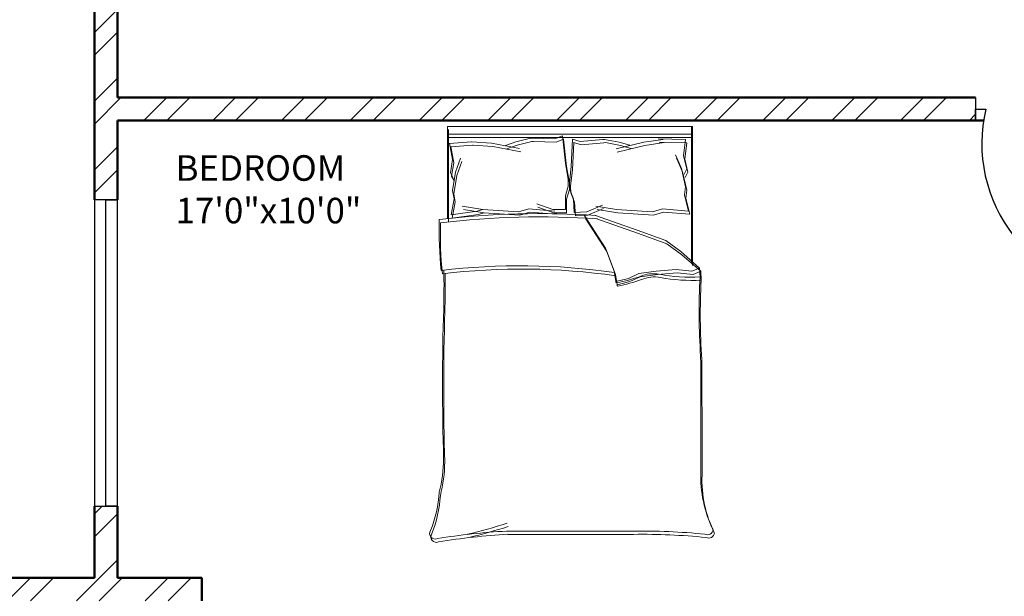
# Model space of a CAD drawing. Units: inches. Extents: x 963 to 2075, y 289 to 2657.
# Tile 60 of 98: x 1149 to 1342, y 2117 to 2230. Entities that reach past the tile are written whole.
import ezdxf

# ---------------------------------------------------------------- set-up
doc = ezdxf.new("R2010")
doc.units = ezdxf.units.IN
for name, color, linetype, lineweight in [('A-AREA-IDEN', 7, 'Continuous', 18), ('A-DOOR', 4, 'Continuous', 25), ('A-FURN', 8, 'Continuous', 18), ('A-GLAZ', 3, 'Continuous', 25), ('A-WALL', 7, 'Continuous', 50), ('A-WALL-PATT', 8, 'Continuous', 13)]:
    doc.layers.add(name, color=color, linetype=linetype, lineweight=lineweight)
doc.styles.get("Standard").update_dxf_attribs({"font": 'arial.ttf'})

# ---------------------------------------------------------------- blocks, each defined once
blk = doc.blocks.new('BED-DOUBLE')
for p, q in [((1236.76, 2450.75), (1254.87, 2450.75)), ((1236.76, 2450.75), (1254.87, 2450.75)), ((1253.34, 2450.75), (1253.34, 2402.96)), ((1253.34, 2450.75), (1253.34, 2402.96)), ((1254.87, 2450.75), (1254.87, 2402.73)), ((1236.12, 2450.52), (1254.23, 2450.52)), ((1236.12, 2450.52), (1254.23, 2450.52)), ((1237.61, 2444.71), (1236.89, 2449.81)), ((1236.89, 2449.81), (1240.07, 2449.23)), ((1237.61, 2444.71), (1236.89, 2449.81)), ((1236.89, 2449.81), (1240.07, 2449.23)), ((1238.25, 2444.94), (1237.53, 2450.04)), ((1237.53, 2450.04), (1240.71, 2449.46)), ((1238.25, 2444.94), (1237.53, 2450.04)), ((1237.53, 2450.04), (1240.71, 2449.46)), ((1240.07, 2449.23), (1241.66, 2449.52)), ((1240.07, 2449.23), (1241.66, 2449.52)), ((1240.71, 2449.46), (1242.3, 2449.75)), ((1240.71, 2449.46), (1242.3, 2449.75)), ((1241.66, 2449.52), (1245.28, 2448.94)), ((1241.66, 2449.52), (1245.28, 2448.94)), ((1242.3, 2449.75), (1245.92, 2449.17)), ((1242.3, 2449.75), (1245.92, 2449.17)), ((1245.13, 2449.96), (1244.12, 2449.38)), ((1245.13, 2449.96), (1244.12, 2449.38)), ((1245.77, 2450.18), (1244.76, 2449.61)), ((1245.77, 2450.18), (1244.76, 2449.61)), ((1247.74, 2449.52), (1245.13, 2449.96)), ((1247.74, 2449.52), (1245.13, 2449.96)), ((1245.28, 2448.94), (1248.02, 2447.93)), ((1245.28, 2448.94), (1248.02, 2447.93)), ((1248.37, 2449.75), (1245.77, 2450.18)), ((1248.37, 2449.75), (1245.77, 2450.18)), ((1245.92, 2449.17), (1248.66, 2448.16)), ((1245.92, 2449.17), (1248.66, 2448.16)), ((1250.92, 2450.1), (1247.74, 2449.52)), ((1250.92, 2450.1), (1247.74, 2449.52)), ((1251.56, 2450.33), (1248.37, 2449.75)), ((1251.56, 2450.33), (1248.37, 2449.75)), ((1250.89, 2450.1), (1251.22, 2445.82)), ((1250.89, 2450.1), (1251.22, 2445.82)), ((1251.53, 2450.32), (1251.86, 2446.04)), ((1251.53, 2450.32), (1251.86, 2446.04)), ((1252.7, 2450.52), (1252.7, 2402.73)), ((1252.7, 2450.52), (1252.7, 2402.73)), ((1238.6, 2447.61), (1237.94, 2443.58)), ((1238.6, 2447.61), (1237.94, 2443.58)), ((1239.24, 2447.84), (1238.58, 2443.81)), ((1239.24, 2447.84), (1238.58, 2443.81)), ((1238.58, 2443.81), (1238.25, 2444.94)), ((1238.58, 2443.81), (1238.25, 2444.94)), ((1251.21, 2445.71), (1250.92, 2441.89)), ((1251.21, 2445.71), (1250.92, 2441.89)), ((1251.22, 2445.82), (1251.21, 2445.71)), ((1251.22, 2445.82), (1251.21, 2445.71)), ((1251.84, 2445.94), (1251.56, 2442.11)), ((1251.84, 2445.94), (1251.56, 2442.11)), ((1251.86, 2446.04), (1251.84, 2445.94)), ((1251.86, 2446.04), (1251.84, 2445.94)), ((1237.94, 2443.58), (1237.51, 2436.57)), ((1237.94, 2443.58), (1237.51, 2436.57)), ((1237.94, 2443.58), (1237.61, 2444.71)), ((1237.94, 2443.58), (1237.61, 2444.71)), ((1238.58, 2443.81), (1238.15, 2436.8)), ((1238.58, 2443.81), (1238.15, 2436.8)), ((1250.92, 2441.89), (1249.9, 2436.39)), ((1250.92, 2441.89), (1249.9, 2436.39)), ((1251.56, 2442.11), (1250.54, 2436.62)), ((1251.56, 2442.11), (1250.54, 2436.62)), ((1175.63, 2439.16), (1175.63, 2414.55)), ((1175.63, 2439.16), (1175.63, 2414.55)), ((1250.48, 2439.14), (1251.21, 2437.12)), ((1250.48, 2439.14), (1251.21, 2437.12)), ((1251.12, 2439.37), (1251.84, 2437.34)), ((1251.12, 2439.37), (1251.84, 2437.34)), ((1174.99, 2438.93), (1174.99, 2414.32)), ((1174.99, 2438.93), (1174.99, 2414.32)), ((1251.21, 2437.12), (1251.93, 2434.22)), ((1251.21, 2437.12), (1251.93, 2434.23)), ((1251.84, 2437.34), (1252.57, 2434.45)), ((1251.84, 2437.34), (1252.57, 2434.45)), ((1237.51, 2436.57), (1238.06, 2434.61)), ((1237.51, 2436.57), (1238.06, 2434.61)), ((1238.15, 2436.8), (1238.7, 2434.84)), ((1238.15, 2436.8), (1238.7, 2434.84)), ((1238.06, 2434.61), (1237.66, 2429.48)), ((1238.06, 2434.61), (1237.66, 2429.48)), ((1238.7, 2434.84), (1238.3, 2429.71)), ((1238.7, 2434.84), (1238.3, 2429.71)), ((1238.61, 2430.12), (1239.7, 2433.26)), ((1238.61, 2430.12), (1239.7, 2433.26)), ((1251.93, 2433.9), (1251.78, 2429.46)), ((1251.93, 2433.9), (1251.78, 2429.46)), ((1251.93, 2434.23), (1251.93, 2433.9)), ((1251.93, 2434.22), (1251.93, 2433.9)), ((1252.57, 2434.13), (1252.42, 2429.69)), ((1252.57, 2434.13), (1252.42, 2429.69)), ((1252.57, 2434.45), (1252.57, 2434.13)), ((1252.57, 2434.45), (1252.57, 2434.13)), ((1237.97, 2429.89), (1239.06, 2433.04)), ((1237.97, 2429.89), (1239.06, 2433.04)), ((1237.97, 2427.43), (1237.97, 2429.89)), ((1237.97, 2427.43), (1237.97, 2429.89)), ((1238.61, 2427.66), (1238.61, 2430.12)), ((1238.61, 2427.66), (1238.61, 2430.12)), ((1251.78, 2429.46), (1252.36, 2428.01)), ((1251.78, 2429.46), (1252.36, 2428.01)), ((1252.42, 2429.69), (1253, 2428.24)), ((1252.42, 2429.69), (1253, 2428.24)), ((1240.65, 2427.43), (1237.97, 2427.43)), ((1240.65, 2427.43), (1237.97, 2427.43)), ((1241.29, 2427.66), (1238.61, 2427.66)), ((1241.29, 2427.66), (1238.61, 2427.66)), ((1242.53, 2426.86), (1240.65, 2427.43)), ((1242.53, 2426.86), (1240.65, 2427.43)), ((1243.17, 2427.08), (1241.29, 2427.66)), ((1243.17, 2427.08), (1241.29, 2427.66)), ((1247.01, 2427.43), (1243.83, 2426.86)), ((1247.01, 2427.43), (1243.83, 2426.86)), ((1247.65, 2427.66), (1244.47, 2427.08)), ((1247.65, 2427.66), (1244.47, 2427.08)), ((1252.36, 2428.01), (1247.01, 2427.43)), ((1252.36, 2428.01), (1247.01, 2427.43)), ((1253, 2428.24), (1247.65, 2427.66)), ((1253, 2428.24), (1247.65, 2427.66)), ((1240.02, 2425.86), (1237.34, 2425.7)), ((1240.02, 2425.86), (1237.34, 2425.7)), ((1237.34, 2425.7), (1237.49, 2423.24)), ((1237.34, 2425.7), (1237.49, 2423.24)), ((1240.66, 2426.09), (1237.98, 2425.93)), ((1240.66, 2426.09), (1237.98, 2425.93)), ((1237.98, 2425.93), (1238.13, 2423.47)), ((1237.98, 2425.93), (1238.13, 2423.47)), ((1241.86, 2426.56), (1240.02, 2425.86)), ((1241.86, 2426.56), (1240.02, 2425.86)), ((1242.49, 2426.79), (1240.66, 2426.09)), ((1242.49, 2426.79), (1240.66, 2426.09)), ((1243.15, 2426.64), (1241.86, 2426.56)), ((1243.15, 2426.64), (1241.86, 2426.56)), ((1243.79, 2426.87), (1242.49, 2426.79)), ((1243.79, 2426.87), (1242.49, 2426.79)), ((1243.83, 2426.86), (1242.53, 2426.86)), ((1243.83, 2426.86), (1242.53, 2426.86)), ((1246.37, 2426.26), (1243.15, 2426.64)), ((1246.37, 2426.26), (1243.15, 2426.64)), ((1244.47, 2427.08), (1243.17, 2427.08)), ((1244.47, 2427.08), (1243.17, 2427.08)), ((1247, 2426.49), (1243.79, 2426.87)), ((1247, 2426.49), (1243.79, 2426.87)), ((1251.74, 2426.02), (1246.37, 2426.26)), ((1251.74, 2426.02), (1246.37, 2426.26)), ((1252.38, 2426.25), (1247, 2426.49)), ((1252.38, 2426.25), (1247, 2426.49)), ((1251.25, 2424.54), (1251.74, 2426.02)), ((1251.25, 2424.54), (1251.74, 2426.02)), ((1251.89, 2424.77), (1252.38, 2426.25)), ((1251.89, 2424.77), (1252.38, 2426.25)), ((1236.85, 2423.74), (1230.36, 2419.55)), ((1236.85, 2423.74), (1230.36, 2419.55)), ((1237.49, 2423.96), (1231, 2419.77)), ((1237.49, 2423.96), (1231, 2419.77)), ((1251.68, 2420.11), (1251.25, 2424.54)), ((1251.68, 2420.11), (1251.25, 2424.54)), ((1252.31, 2420.34), (1251.89, 2424.77)), ((1252.31, 2420.34), (1251.89, 2424.77)), ((1233.92, 2413.35), (1236.85, 2421.69)), ((1233.92, 2413.35), (1236.85, 2421.69)), ((1234.56, 2413.58), (1237.49, 2421.92)), ((1234.56, 2413.58), (1237.49, 2421.92)), ((1237.49, 2423.24), (1238.78, 2420.17)), ((1237.49, 2423.24), (1238.78, 2420.17)), ((1238.13, 2423.47), (1239.42, 2420.4)), ((1238.13, 2423.47), (1239.42, 2420.4)), ((1239.24, 2421.66), (1238.58, 2417.63)), ((1239.24, 2421.66), (1238.58, 2417.63)), ((1231, 2419.77), (1226.51, 2418.07)), ((1231, 2419.77), (1226.51, 2418.07)), ((1238.6, 2421.43), (1237.94, 2417.4)), ((1238.6, 2421.43), (1237.94, 2417.4)), ((1251.15, 2416.86), (1251.7, 2419.79)), ((1251.15, 2416.86), (1251.7, 2419.79)), ((1251.7, 2419.79), (1251.68, 2420.11)), ((1251.7, 2419.79), (1251.68, 2420.11)), ((1251.79, 2417.09), (1252.33, 2420.02)), ((1251.79, 2417.09), (1252.33, 2420.02)), ((1252.33, 2420.02), (1252.31, 2420.34)), ((1252.33, 2420.02), (1252.31, 2420.34)), ((1225.87, 2417.84), (1223.86, 2417.53)), ((1225.87, 2417.84), (1223.86, 2417.53)), ((1226.51, 2418.07), (1224.49, 2417.76)), ((1226.51, 2418.07), (1224.49, 2417.76)), ((1230.36, 2419.55), (1225.87, 2417.84)), ((1230.36, 2419.55), (1225.87, 2417.84)), ((1223.86, 2417.53), (1224.47, 2415.05)), ((1223.86, 2417.53), (1224.47, 2415.05)), ((1224.49, 2417.76), (1225.11, 2415.28)), ((1224.49, 2417.76), (1225.11, 2415.28)), ((1237.94, 2417.4), (1237.51, 2410.39)), ((1237.94, 2417.4), (1237.51, 2410.39)), ((1238.58, 2417.63), (1238.15, 2410.62)), ((1238.58, 2417.63), (1238.15, 2410.62)), ((1251.16, 2412.08), (1249.81, 2417.5)), ((1251.16, 2412.08), (1249.81, 2417.5)), ((1251.8, 2412.31), (1250.45, 2417.73)), ((1251.8, 2412.31), (1250.45, 2417.73)), ((1250.56, 2414.79), (1251.15, 2416.86)), ((1250.56, 2414.79), (1251.15, 2416.86)), ((1251.2, 2415.02), (1251.79, 2417.09)), ((1251.2, 2415.02), (1251.79, 2417.09)), ((1224.47, 2415.05), (1225.4, 2413.04)), ((1224.47, 2415.05), (1225.4, 2413.04)), ((1225.11, 2415.28), (1226.04, 2413.27)), ((1225.11, 2415.28), (1226.04, 2413.27)), ((1225.4, 2413.04), (1225.87, 2409.63)), ((1225.4, 2413.04), (1225.87, 2409.63)), ((1226.04, 2413.27), (1226.51, 2409.86)), ((1226.04, 2413.27), (1226.51, 2409.86)), ((1231.9, 2407.77), (1233.92, 2413.35)), ((1231.9, 2407.78), (1233.92, 2413.35)), ((1232.54, 2408), (1234.56, 2413.58)), ((1232.54, 2408), (1234.56, 2413.58)), ((1251.69, 2408.28), (1251.16, 2412.08)), ((1251.69, 2408.28), (1251.16, 2412.08)), ((1252.33, 2408.51), (1251.8, 2412.31)), ((1252.33, 2408.51), (1251.8, 2412.31)), ((1237.51, 2410.39), (1238.06, 2408.43)), ((1237.51, 2410.39), (1238.06, 2408.43)), ((1238.15, 2410.62), (1238.7, 2408.66)), ((1238.15, 2410.62), (1238.7, 2408.66)), ((1225.87, 2409.63), (1226.18, 2405.76)), ((1225.87, 2409.63), (1226.18, 2405.76)), ((1226.51, 2409.86), (1226.82, 2405.99)), ((1226.51, 2409.86), (1226.82, 2405.99)), ((1238.06, 2408.43), (1237.66, 2403.3)), ((1238.06, 2408.43), (1237.66, 2403.3)), ((1238.7, 2408.66), (1238.3, 2403.52)), ((1238.7, 2408.66), (1238.3, 2403.52)), ((1251.68, 2403.88), (1251.77, 2409.29)), ((1251.68, 2403.88), (1251.77, 2409.28)), ((1251.77, 2409.29), (1251.69, 2408.28)), ((1251.77, 2409.28), (1251.69, 2408.28)), ((1252.31, 2404.11), (1252.41, 2409.51)), ((1252.31, 2404.11), (1252.41, 2409.51)), ((1252.41, 2409.51), (1252.33, 2408.51)), ((1252.41, 2409.51), (1252.33, 2408.51)), ((1229.74, 2404.83), (1231.9, 2407.78)), ((1229.74, 2404.83), (1231.9, 2407.77)), ((1230.38, 2405.06), (1232.54, 2408)), ((1230.38, 2405.06), (1232.54, 2408)), ((1226.18, 2405.76), (1225.87, 2402.66)), ((1226.18, 2405.76), (1225.87, 2402.66)), ((1226.49, 2401.13), (1229.74, 2404.83)), ((1226.49, 2401.13), (1229.74, 2404.83)), ((1226.82, 2405.99), (1226.51, 2402.89)), ((1226.82, 2405.99), (1226.51, 2402.89)), ((1227.13, 2401.36), (1230.38, 2405.06)), ((1227.13, 2401.36), (1230.38, 2405.06)), ((1238.3, 2403.52), (1241.44, 2404.3)), ((1238.3, 2403.52), (1241.44, 2404.3)), ((1241.44, 2404.3), (1243.04, 2404.11)), ((1241.44, 2404.3), (1243.04, 2404.11)), ((1242.4, 2403.88), (1245.98, 2404.69)), ((1242.4, 2403.88), (1245.98, 2404.69)), ((1243.04, 2404.11), (1246.61, 2404.91)), ((1243.04, 2404.11), (1246.61, 2404.91)), ((1246.53, 2403.89), (1245.49, 2404.41)), ((1246.53, 2403.89), (1245.49, 2404.41)), ((1245.98, 2404.69), (1248.65, 2405.87)), ((1245.98, 2404.69), (1248.65, 2405.87)), ((1249.1, 2404.49), (1246.53, 2403.89)), ((1249.1, 2404.49), (1246.53, 2403.89)), ((1246.61, 2404.91), (1249.29, 2406.1)), ((1246.61, 2404.91), (1249.29, 2406.09)), ((1252.31, 2404.11), (1249.1, 2404.49)), ((1252.31, 2404.11), (1249.1, 2404.49)), ((1225.87, 2402.66), (1226.49, 2401.13)), ((1225.87, 2402.66), (1226.49, 2401.13)), ((1226.51, 2402.89), (1227.13, 2401.36)), ((1226.51, 2402.89), (1227.13, 2401.36)), ((1254.23, 2402.73), (1227.62, 2402.73)), ((1254.23, 2402.73), (1227.62, 2402.73)), ((1254.87, 2402.96), (1228.26, 2402.96)), ((1254.87, 2402.96), (1228.26, 2402.96)), ((1237.66, 2403.3), (1240.8, 2404.07)), ((1237.66, 2403.3), (1240.8, 2404.07)), ((1240.8, 2404.07), (1242.4, 2403.88)), ((1240.8, 2404.07), (1242.4, 2403.88)), ((1245.89, 2403.67), (1244.85, 2404.18)), ((1245.89, 2403.67), (1244.85, 2404.18)), ((1248.46, 2404.26), (1245.89, 2403.67)), ((1248.46, 2404.26), (1245.89, 2403.67)), ((1251.68, 2403.88), (1248.46, 2404.26)), ((1251.68, 2403.88), (1248.46, 2404.26)), ((1254.87, 2402.73), (1254.23, 2402.73)), ((1224.74, 2401.05), (1226.49, 2401.13, 3.87)), ((1224.74, 2401.05), (1226.49, 2401.13, 3.87)), ((1225.38, 2401.28), (1227.13, 2401.36, 3.87)), ((1225.38, 2401.28), (1227.13, 2401.36, 3.87))]:
    blk.add_line(p, q)
for centre, radius, start, end in [((1174.51, 2452.91), 1.09, 56.1736, 203.4781), ((1174.51, 2452.91), 1.09, 56.1736, 203.4781), ((1053.4, 2432.57), 121.76, 2.9958, 9.4091), ((1053.4, 2432.57), 121.76, 2.9958, 9.4091), ((1175.15, 2453.14), 1.09, 56.1736, 203.4781), ((1175.15, 2453.14), 1.09, 56.1736, 203.4781), ((1054.03, 2432.8), 121.76, 2.9958, 9.4091), ((1054.03, 2432.8), 121.76, 2.9958, 9.4091), ((1183.96, 2475.65), 23.56, 247.9751, 266.652), ((1183.96, 2475.65), 23.56, 247.9751, 266.652), ((1184.6, 2475.88), 23.56, 247.9751, 266.652), ((1184.6, 2475.88), 23.56, 247.9751, 266.652), ((1189.72, 2480.89), 29.63, 256.0648, 268.9113), ((1189.72, 2480.89), 29.63, 256.0648, 268.9113), ((1190.36, 2481.12), 29.63, 256.0648, 268.9113), ((1190.36, 2481.12), 29.63, 256.0648, 268.9113), ((1203.62, 1969.17), 482.31, 88.2277, 91.7185), ((1203.62, 1969.17), 482.31, 88.2277, 91.7185), ((1204.26, 1969.4), 482.31, 88.2277, 91.7185), ((1204.26, 1969.4), 482.31, 88.2277, 91.7185), ((1223.06, 2621.3), 170.11, 268.4762, 271.0082), ((1223.06, 2621.3), 170.11, 268.4762, 271.0082), ((1223.7, 2621.53), 170.11, 268.4762, 271.0082), ((1223.7, 2621.53), 170.11, 268.4762, 271.0082), ((1097.92, 2436.24), 129.02, 351.7845, 6.9006), ((1097.92, 2436.24), 129.02, 351.7845, 6.9006), ((1234.14, 2368.83), 83.31, 88.7218, 95.604), ((1234.14, 2368.83), 83.31, 88.7218, 95.604), ((1098.56, 2436.47), 129.02, 351.7845, 6.9006), ((1098.56, 2436.47), 129.02, 351.7845, 6.9006), ((1234.78, 2369.06), 83.31, 88.7218, 95.604), ((1234.78, 2369.06), 83.31, 88.7218, 95.604), ((1072.18, 2432.64), 164.97, 356.0865, 6.7821), ((1072.18, 2432.64), 164.97, 356.0865, 6.7821), ((1072.82, 2432.86), 164.97, 356.0865, 6.7821), ((1072.82, 2432.86), 164.97, 356.0865, 6.7821), ((1278.58, 2471.44), 106.46, 193.3832, 197.7053), ((1278.58, 2471.44), 106.46, 193.3832, 197.7053), ((1277.94, 2471.22), 106.46, 193.3832, 197.7053), ((1277.94, 2471.22), 106.46, 193.3832, 197.7053), ((1224.43, 2417.59), 0.185, 70.2464, 181.1377), ((1224.43, 2417.59), 0.185, 70.2464, 181.1377), ((1223.79, 2417.36), 0.185, 70.2464, 181.1377), ((1223.79, 2417.36), 0.185, 70.2464, 181.1377), ((1252.75, 2422.84), 29.65, 190.6617, 199.8806), ((1252.75, 2422.84), 29.65, 190.6617, 199.8806), ((1253.39, 2423.07), 29.65, 190.6617, 199.8806), ((1253.39, 2423.07), 29.65, 190.6617, 199.8806), ((1041.96, 2412.84), 133.04, 354.4998, 0.6351), ((1041.96, 2412.84), 133.04, 354.4998, 0.6351), ((1042.6, 2413.07), 133.04, 354.4998, 0.6351), ((1042.6, 2413.07), 133.04, 354.4998, 0.6351), ((1219.17, 2410.25), 6.22, 348.6608, 23.7384), ((1219.17, 2410.25), 6.22, 348.6608, 23.7384), ((1219.81, 2410.48), 6.22, 348.6608, 23.7384), ((1219.81, 2410.48), 6.22, 348.6608, 23.7384), ((1260.89, 2402.67), 36.18, 169.8763, 182.5657), ((1260.89, 2402.67), 36.18, 169.8763, 182.5657), ((1261.53, 2402.9), 36.18, 169.8763, 182.5657), ((1261.53, 2402.9), 36.18, 169.8763, 182.5657), ((1185.57, 2377.84), 23.07, 87.4714, 116.4681), ((1185.57, 2377.84), 23.07, 87.4714, 116.4681), ((1186.21, 2378.07), 23.07, 87.4714, 116.4681), ((1186.21, 2378.07), 23.07, 87.4714, 116.4681), ((1186.41, 6962.74), 4561.86, 270.00217, 270.28689), ((1186.41, 6962.74), 4561.86, 270.00217, 270.28689), ((1187.05, 6962.97), 4561.86, 270.00217, 270.28689), ((1187.05, 6962.97), 4561.86, 270.00217, 270.28689), ((1217.92, 2271.73), 129.5, 86.9791, 93.8365), ((1217.92, 2271.73), 129.5, 86.9791, 93.8365), ((1218.56, 2271.96), 129.5, 86.9791, 93.8365), ((1218.56, 2271.96), 129.5, 86.9791, 93.8365), ((1175.36, 2399.58), 1.1, 152.6588, 266.02), ((1175.36, 2399.58), 1.1, 152.6588, 266.02), ((1176, 2399.81), 1.1, 152.6588, 266.02), ((1176, 2399.81), 1.1, 152.6588, 266.02)]:
    blk.add_arc(centre, radius, start, end)

msp = doc.modelspace()

# ---------------------------------------------------------------- hatches: boundary and pattern name
at = {"layer": 'A-WALL-PATT'}
h = msp.add_hatch(dxfattribs=at)
h.set_pattern_fill('ANSI32', color=256)
h.paths.add_polyline_path([(1296.92, 2558.32), (1203.92, 2558.32), (1203.92, 2493.82), (1191.53, 2493.82), (1191.53, 2489.32), (1211.06, 2489.32), (1211.06, 2492.02), (1211.06, 2493.82), (1208.42, 2493.82), (1208.42, 2553.82), (1292.42, 2553.82), (1292.42, 2538.86), (1296.92, 2538.86)])
h.paths.add_polyline_path([(1442.42, 2558.32), (1349.42, 2558.32), (1349.42, 2538.94), (1353.92, 2538.94), (1353.92, 2553.82), (1437.92, 2553.82), (1437.92, 2493.82), (1434.54, 2493.82), (1434.54, 2489.32), (1448.31, 2489.32), (1448.31, 2491.57), (1448.31, 2493.82), (1442.42, 2493.82)])
h.paths.add_polyline_path([(1415.55, 2491.57), (1415.55, 2493.82), (1340.94, 2493.82), (1340.94, 2489.32), (1371.92, 2489.32), (1371.92, 2378.32), (1367.6, 2378.32), (1367.6, 2373.82), (1371.92, 2373.82), (1371.92, 2355.19), (1376.42, 2355.19), (1376.42, 2489.32), (1415.55, 2489.32)])
h.paths.add_polyline_path([(1304.94, 2491.57), (1304.94, 2493.82), (1296.92, 2493.82), (1296.92, 2514.86), (1292.42, 2514.86), (1292.42, 2493.82), (1232.81, 2493.82), (1232.81, 2489.32), (1256.42, 2489.32), (1256.42, 2327.32), (1253.71, 2327.32), (1253.71, 2322.82), (1328.42, 2322.82), (1328.42, 2331.15), (1323.92, 2331.15), (1323.92, 2327.32), (1260.92, 2327.32), (1260.92, 2373.82), (1323.92, 2373.82), (1323.92, 2357.81), (1328.42, 2357.81), (1328.42, 2373.82), (1346.01, 2373.82), (1346.01, 2376.07), (1346.01, 2378.32), (1260.92, 2378.32), (1260.92, 2489.32), (1304.94, 2489.32)])
h.paths.add_polyline_path([(1226.65, 2327.32), (1124.42, 2327.32), (1124.42, 2347.45), (1119.92, 2347.45), (1119.92, 2322.82), (1163.42, 2322.82), (1163.42, 2305.43), (1165.67, 2305.43), (1167.92, 2305.43), (1167.92, 2322.82), (1226.65, 2322.82), (1226.65, 2325.07)])
h.paths.add_polyline_path([(1095.92, 2489.32), (1124.42, 2489.32), (1131.53, 2489.32), (1131.53, 2491.57), (1131.53, 2493.82), (1119.92, 2493.82), (1091.42, 2493.82), (1091.42, 2417.32), (1095.92, 2417.32), (1119.92, 2417.32), (1119.92, 2407.45), (1124.42, 2407.45), (1124.42, 2421.82), (1095.92, 2421.82)])
h.paths.add_polyline_path([(1512.92, 2558.32), (1508.42, 2558.32), (1508.42, 2493.82), (1503.4, 2493.82), (1503.4, 2489.32), (1508.42, 2489.32), (1508.42, 2327.32), (1376.42, 2327.32), (1376.42, 2330.27), (1371.92, 2330.27), (1371.92, 2298.74), (1376.42, 2298.74), (1376.42, 2322.82), (1508.42, 2322.82), (1508.42, 2165.32), (1504.26, 2165.32), (1504.26, 2160.82), (1508.42, 2160.82), (1508.42, 2108.32), (1512.92, 2108.32), (1512.92, 2160.82), (1516.18, 2160.82), (1516.18, 2163.07), (1516.18, 2165.32), (1512.92, 2165.32), (1512.92, 2322.82), (1644.92, 2322.82), (1644.92, 2298.74), (1649.42, 2298.74), (1649.42, 2322.82), (1649.42, 2330.94), (1647.17, 2330.94), (1644.92, 2330.94), (1644.92, 2327.32), (1512.92, 2327.32), (1512.92, 2489.32), (1516.76, 2489.32), (1516.76, 2491.57), (1516.76, 2493.82), (1512.92, 2493.82)])
h.paths.add_polyline_path([(1671.92, 2558.32), (1578.92, 2558.32), (1578.92, 2493.82), (1573.53, 2493.82), (1573.53, 2489.32), (1586.54, 2489.32), (1586.54, 2491.57), (1586.54, 2493.82), (1583.42, 2493.82), (1583.42, 2553.82), (1667.42, 2553.82), (1667.42, 2541.11), (1671.92, 2541.11)])
h.paths.add_polyline_path([(1681.26, 2493.82), (1671.92, 2493.82), (1671.92, 2517.11), (1667.42, 2517.11), (1667.42, 2493.82), (1610.22, 2493.82), (1610.22, 2489.32), (1644.92, 2489.32), (1644.92, 2357.87), (1649.42, 2357.87), (1649.42, 2373.82), (1652.2, 2373.82), (1652.2, 2375.83), (1652.2, 2378.32), (1649.42, 2378.32), (1649.42, 2489.32), (1681.26, 2489.32), (1681.26, 2491.57)])
h.paths.add_polyline_path([(1821.92, 2558.32), (1728.92, 2558.32), (1728.92, 2541), (1733.42, 2541), (1733.42, 2553.82), (1817.42, 2553.82), (1817.42, 2493.82), (1813.51, 2493.82), (1813.51, 2489.32), (1830.08, 2489.32), (1830.08, 2491.57), (1830.08, 2493.82), (1821.92, 2493.82)])
h.paths.add_polyline_path([(1794.24, 2493.82), (1717.26, 2493.82), (1717.26, 2489.32), (1760.42, 2489.32), (1760.42, 2378.32), (1674.4, 2378.32), (1674.4, 2373.82), (1692.92, 2373.82), (1692.92, 2356.95), (1697.42, 2356.95), (1697.42, 2373.82), (1760.42, 2373.82), (1760.42, 2327.32), (1697.42, 2327.32), (1697.42, 2333.34), (1692.92, 2333.34), (1692.92, 2322.82), (1768.04, 2322.82), (1768.04, 2325.07), (1768.04, 2327.32), (1764.92, 2327.32), (1764.92, 2489.32), (1794.24, 2489.32)])
h.paths.add_polyline_path([(1733.42, 2517), (1728.92, 2517), (1728.92, 2493.82), (1733.42, 2493.82)], flags=17)
h.paths.add_polyline_path([(1929.92, 2493.82), (1890.08, 2493.82), (1890.08, 2489.32), (1896.92, 2489.32), (1925.42, 2489.32), (1925.42, 2421.82), (1896.92, 2421.82), (1896.92, 2408.32), (1901.42, 2408.32), (1901.42, 2417.32), (1925.42, 2417.32), (1929.92, 2417.32)])
h.paths.add_polyline_path([(1901.42, 2348.32), (1896.92, 2348.32), (1896.92, 2327.32), (1800.42, 2327.32), (1800.42, 2322.82), (1853.42, 2322.82), (1853.42, 2309.45), (1857.92, 2309.45), (1857.92, 2322.82), (1901.42, 2322.82)])
h.paths.add_polyline_path([(1857.92, 2249.45), (1853.42, 2249.45), (1853.42, 2214.82), (1686.31, 2214.82), (1686.31, 2210.32), (1853.42, 2210.32), (1853.42, 2202.13), (1857.92, 2202.13), (1857.92, 2210.32)])
h.paths.add_polyline_path([(1857.92, 2142.13), (1853.42, 2142.13), (1853.42, 2115.42), (1841.42, 2115.42), (1841.42, 2088.53), (1841.42, 2046.95), (1845.92, 2046.95), (1845.92, 2110.92), (1905.92, 2110.92), (1905.92, 2092.52), (1910.42, 2092.52), (1910.42, 2115.42), (1857.92, 2115.42)])
h.paths.add_polyline_path([(1532.44, 1482.34), (1573.46, 1482.34), (1573.46, 1501), (1532.44, 1501)], flags=9)
h.paths.add_polyline_path([(1438.66, 1486.3), (1479.68, 1486.3), (1479.68, 1504.96), (1438.66, 1504.96)], flags=9)
h.paths.add_polyline_path([(1411.22, 1365.31), (1659.14, 1365.31), (1659.14, 1402.4), (1411.22, 1402.4)], flags=9)
h.paths.add_polyline_path([(1185.67, 2296.3), (1248.16, 2296.3), (1248.16, 2314.95), (1185.67, 2314.95)], flags=9)
h.paths.add_polyline_path([(1177.31, 2187.35), (1216.15, 2187.35), (1216.15, 2206.01), (1177.31, 2206.01)], flags=9)
h.paths.add_polyline_path([(1295.1, 1602.08), (1328.26, 1602.08), (1328.26, 1620.74), (1295.1, 1620.74)], flags=9)
h.paths.add_polyline_path([(1525.13, 2005.99), (1558.39, 2005.99), (1558.39, 2024.65), (1525.13, 2024.65)], flags=9)
h.paths.add_polyline_path([(1459.61, 1977.13), (1472.19, 1977.13), (1472.19, 1987.43), (1459.61, 1987.43)], flags=9)
h.paths.add_polyline_path([(1467.81, 2053.68), (1480.02, 2053.68), (1480.02, 2063.98), (1467.81, 2063.98)], flags=9)
h.paths.add_polyline_path([(1555.18, 2119.02), (1584.56, 2119.02), (1584.56, 2137.68), (1555.18, 2137.68)], flags=25)
h.paths.add_polyline_path([(1405.39, 2115.29), (1444.48, 2115.29), (1444.48, 2133.95), (1405.39, 2133.95)], flags=25)
h.paths.add_polyline_path([(1698.48, 2004.26), (1727.69, 2004.26), (1727.69, 2022.92), (1698.48, 2022.92)], flags=9)
h.paths.add_polyline_path([(1612.16, 1972.86), (1629.02, 1972.86), (1629.02, 1983.16), (1612.16, 1983.16)], flags=9)
h.paths.add_polyline_path([(1608.29, 2060.04), (1625.15, 2060.04), (1625.15, 2070.34), (1608.29, 2070.34)], flags=9)
h.paths.add_polyline_path([(1527.95, 1684.4), (1566.79, 1684.4), (1566.79, 1703.06), (1527.95, 1703.06)], flags=9)
h.paths.add_polyline_path([(1422.79, 1683.59), (1461.63, 1683.59), (1461.63, 1702.25), (1422.79, 1702.25)], flags=9)
h.paths.add_polyline_path([(1531.26, 1732.46), (1574.01, 1732.46), (1574.01, 1751.12), (1531.26, 1751.12)], flags=9)
h.paths.add_polyline_path([(1402.87, 1732.85), (1439.8, 1732.85), (1439.8, 1751.5), (1402.87, 1751.5)], flags=9)
h.paths.add_polyline_path([(1243.12, 1923.13), (1281.96, 1923.13), (1281.96, 1941.79), (1243.12, 1941.79)], flags=9)
h.paths.add_polyline_path([(1181.75, 1792.27), (1244.24, 1792.27), (1244.24, 1810.93), (1181.75, 1810.93)], flags=9)
h.paths.add_polyline_path([(1265.82, 1670.3), (1316.07, 1670.3), (1316.07, 1688.96), (1265.82, 1688.96)], flags=9)
h.paths.add_polyline_path([(1140.26, 1676.05), (1179.1, 1676.05), (1179.1, 1694.71), (1140.26, 1694.71)], flags=9)
h.paths.add_polyline_path([(1107.49, 1490.89), (1143.37, 1490.89), (1143.37, 1509.55), (1107.49, 1509.55)], flags=9)
h.paths.add_polyline_path([(1217.58, 1483.9), (1246.74, 1483.9), (1246.74, 1502.56), (1217.58, 1502.56)], flags=9)
h.paths.add_polyline_path([(1389.21, 1486.92), (1418.37, 1486.92), (1418.37, 1505.58), (1389.21, 1505.58)], flags=9)
h.paths.add_polyline_path([(1672.21, 1602.08), (1705.37, 1602.08), (1705.37, 1620.74), (1672.21, 1620.74)], flags=9)
h.paths.add_polyline_path([(1752.08, 1522.64), (1781.24, 1522.64), (1781.24, 1541.3), (1752.08, 1541.3)], flags=9)
h.paths.add_polyline_path([(1848.27, 1491.26), (1884.16, 1491.26), (1884.16, 1509.92), (1848.27, 1509.92)], flags=9)
h.paths.add_polyline_path([(1822.47, 1685.62), (1861.31, 1685.62), (1861.31, 1704.28), (1822.47, 1704.28)], flags=9)
h.paths.add_polyline_path([(1713.19, 1672.23), (1763.44, 1672.23), (1763.44, 1690.89), (1713.19, 1690.89)], flags=9)
h.paths.add_polyline_path([(1736.62, 1790.58), (1799.11, 1790.58), (1799.11, 1809.24), (1736.62, 1809.24)], flags=9)
h.paths.add_polyline_path([(1691.49, 1916.36), (1730.33, 1916.36), (1730.33, 1935.01), (1691.49, 1935.01)], flags=9)
h.paths.add_polyline_path([(1764.87, 1973.92), (1794.31, 1973.92), (1794.31, 1992.58), (1764.87, 1992.58)], flags=9)
h.paths.add_polyline_path([(1767.85, 2034.02), (1797.29, 2034.02), (1797.29, 2052.67), (1767.85, 2052.67)], flags=9)
h.paths.add_polyline_path([(1851.59, 2060.33), (1880.75, 2060.33), (1880.75, 2078.99), (1851.59, 2078.99)], flags=25)
h.paths.add_polyline_path([(1688.49, 2086.87), (1727.33, 2086.87), (1727.33, 2105.53), (1688.49, 2105.53)], flags=9)
h.paths.add_polyline_path([(1537.74, 2293.58), (1580.49, 2293.58), (1580.49, 2312.24), (1537.74, 2312.24)], flags=25)
h.paths.add_polyline_path([(1425.59, 2296.11), (1468.34, 2296.11), (1468.34, 2314.77), (1425.59, 2314.77)], flags=25)
h.paths.add_polyline_path([(1278.52, 2004.18), (1307.72, 2004.18), (1307.72, 2022.84), (1278.52, 2022.84)], flags=9)
h.paths.add_polyline_path([(1193.28, 1973.63), (1222.72, 1973.63), (1222.72, 1992.29), (1193.28, 1992.29)], flags=9)
h.paths.add_polyline_path([(1192.41, 2040.58), (1221.84, 2040.58), (1221.84, 2059.23), (1192.41, 2059.23)], flags=9)
h.paths.add_polyline_path([(1130.6, 1951.39), (1159.76, 1951.39), (1159.76, 1970.05), (1130.6, 1970.05)], flags=9)
h.paths.add_polyline_path([(1132.83, 2052.49), (1161.98, 2052.49), (1161.98, 2071.15), (1132.83, 2071.15)], flags=9)
h.paths.add_polyline_path([(1265.13, 2334.62), (1315.38, 2334.62), (1315.38, 2353.28), (1265.13, 2353.28)], flags=25)
h.paths.add_polyline_path([(1136.74, 2330.79), (1175.58, 2330.79), (1175.58, 2349.44), (1136.74, 2349.44)], flags=9)
h.paths.add_polyline_path([(1287.42, 2417.2), (1320.58, 2417.2), (1320.58, 2435.86), (1287.42, 2435.86)], flags=25)
h.paths.add_polyline_path([(1430.99, 2329.16), (1469.83, 2329.16), (1469.83, 2347.82), (1430.99, 2347.82)], flags=25)
h.paths.add_polyline_path([(1525.42, 2329.21), (1564.26, 2329.21), (1564.26, 2347.87), (1525.42, 2347.87)], flags=25)
h.paths.add_polyline_path([(1684.52, 2382.8), (1717.68, 2382.8), (1717.68, 2401.46), (1684.52, 2401.46)], flags=25)
h.paths.add_polyline_path([(1704.81, 2340.29), (1755.05, 2340.29), (1755.05, 2358.95), (1704.81, 2358.95)], flags=25)
h.paths.add_polyline_path([(1694.11, 2287.76), (1756.6, 2287.76), (1756.6, 2306.41), (1694.11, 2306.41)], flags=9)
h.paths.add_polyline_path([(1815.78, 2329.86), (1854.62, 2329.86), (1854.62, 2348.52), (1815.78, 2348.52)], flags=9)
h.paths.add_polyline_path([(1842.87, 2514.26), (1878.76, 2514.26), (1878.76, 2532.91), (1842.87, 2532.91)], flags=9)
h.paths.add_polyline_path([(1769.51, 2531.45), (1798.67, 2531.45), (1798.67, 2550.1), (1769.51, 2550.1)], flags=25)
h.paths.add_polyline_path([(1594.77, 2518.47), (1623.93, 2518.47), (1623.93, 2537.13), (1594.77, 2537.13)], flags=25)
h.paths.add_polyline_path([(1520.72, 2516.18), (1556.61, 2516.18), (1556.61, 2534.84), (1520.72, 2534.84)], flags=25)
h.paths.add_polyline_path([(1464.46, 2516.69), (1500.34, 2516.69), (1500.34, 2535.35), (1464.46, 2535.35)], flags=25)
h.paths.add_polyline_path([(1365.7, 2528.97), (1394.85, 2528.97), (1394.85, 2547.63), (1365.7, 2547.63)], flags=25)
h.paths.add_polyline_path([(1222.84, 2516.23), (1252, 2516.23), (1252, 2534.89), (1222.84, 2534.89)], flags=25)
h.paths.add_polyline_path([(1104.55, 2509.6), (1140.43, 2509.6), (1140.43, 2528.26), (1104.55, 2528.26)], flags=9)
h = msp.add_hatch(dxfattribs=at)
h.set_pattern_fill('ANSI32', color=256)
h.paths.add_polyline_path([(1335.97, 2212.57), (1335.97, 2214.82), (1167.92, 2214.82), (1167.92, 2245.43), (1163.42, 2245.43), (1163.42, 2210.32), (1163.42, 2194.81), (1167.92, 2194.81), (1167.92, 2210.32), (1335.97, 2210.32)])
h.paths.add_polyline_path([(1532.44, 1482.34), (1573.46, 1482.34), (1573.46, 1501), (1532.44, 1501)], flags=9)
h.paths.add_polyline_path([(1438.66, 1486.3), (1479.68, 1486.3), (1479.68, 1504.96), (1438.66, 1504.96)], flags=9)
h.paths.add_polyline_path([(1411.22, 1365.31), (1659.14, 1365.31), (1659.14, 1402.4), (1411.22, 1402.4)], flags=9)
h.paths.add_polyline_path([(1185.67, 2296.3), (1248.16, 2296.3), (1248.16, 2314.95), (1185.67, 2314.95)], flags=9)
h.paths.add_polyline_path([(1177.31, 2187.35), (1216.15, 2187.35), (1216.15, 2206.01), (1177.31, 2206.01)], flags=9)
h.paths.add_polyline_path([(1295.1, 1602.08), (1328.26, 1602.08), (1328.26, 1620.74), (1295.1, 1620.74)], flags=9)
h.paths.add_polyline_path([(1525.13, 2005.99), (1558.39, 2005.99), (1558.39, 2024.65), (1525.13, 2024.65)], flags=9)
h.paths.add_polyline_path([(1459.61, 1977.13), (1472.19, 1977.13), (1472.19, 1987.43), (1459.61, 1987.43)], flags=9)
h.paths.add_polyline_path([(1467.81, 2053.68), (1480.02, 2053.68), (1480.02, 2063.98), (1467.81, 2063.98)], flags=9)
h.paths.add_polyline_path([(1555.18, 2119.02), (1584.56, 2119.02), (1584.56, 2137.68), (1555.18, 2137.68)], flags=9)
h.paths.add_polyline_path([(1405.39, 2115.29), (1444.48, 2115.29), (1444.48, 2133.95), (1405.39, 2133.95)], flags=9)
h.paths.add_polyline_path([(1698.48, 2004.26), (1727.69, 2004.26), (1727.69, 2022.92), (1698.48, 2022.92)], flags=9)
h.paths.add_polyline_path([(1612.16, 1972.86), (1629.02, 1972.86), (1629.02, 1983.16), (1612.16, 1983.16)], flags=9)
h.paths.add_polyline_path([(1608.29, 2060.04), (1625.15, 2060.04), (1625.15, 2070.34), (1608.29, 2070.34)], flags=9)
h.paths.add_polyline_path([(1527.95, 1684.4), (1566.79, 1684.4), (1566.79, 1703.06), (1527.95, 1703.06)], flags=9)
h.paths.add_polyline_path([(1422.79, 1683.59), (1461.63, 1683.59), (1461.63, 1702.25), (1422.79, 1702.25)], flags=9)
h.paths.add_polyline_path([(1531.26, 1732.46), (1574.01, 1732.46), (1574.01, 1751.12), (1531.26, 1751.12)], flags=9)
h.paths.add_polyline_path([(1402.87, 1732.85), (1439.8, 1732.85), (1439.8, 1751.5), (1402.87, 1751.5)], flags=9)
h.paths.add_polyline_path([(1243.12, 1923.13), (1281.96, 1923.13), (1281.96, 1941.79), (1243.12, 1941.79)], flags=9)
h.paths.add_polyline_path([(1181.75, 1792.27), (1244.24, 1792.27), (1244.24, 1810.93), (1181.75, 1810.93)], flags=9)
h.paths.add_polyline_path([(1265.82, 1670.3), (1316.07, 1670.3), (1316.07, 1688.96), (1265.82, 1688.96)], flags=9)
h.paths.add_polyline_path([(1140.26, 1676.05), (1179.1, 1676.05), (1179.1, 1694.71), (1140.26, 1694.71)], flags=9)
h.paths.add_polyline_path([(1107.49, 1490.89), (1143.37, 1490.89), (1143.37, 1509.55), (1107.49, 1509.55)], flags=9)
h.paths.add_polyline_path([(1217.58, 1483.9), (1246.74, 1483.9), (1246.74, 1502.56), (1217.58, 1502.56)], flags=9)
h.paths.add_polyline_path([(1389.21, 1486.92), (1418.37, 1486.92), (1418.37, 1505.58), (1389.21, 1505.58)], flags=9)
h.paths.add_polyline_path([(1672.21, 1602.08), (1705.37, 1602.08), (1705.37, 1620.74), (1672.21, 1620.74)], flags=9)
h.paths.add_polyline_path([(1752.08, 1522.64), (1781.24, 1522.64), (1781.24, 1541.3), (1752.08, 1541.3)], flags=9)
h.paths.add_polyline_path([(1848.27, 1491.26), (1884.16, 1491.26), (1884.16, 1509.92), (1848.27, 1509.92)], flags=9)
h.paths.add_polyline_path([(1822.47, 1685.62), (1861.31, 1685.62), (1861.31, 1704.28), (1822.47, 1704.28)], flags=9)
h.paths.add_polyline_path([(1713.19, 1672.23), (1763.44, 1672.23), (1763.44, 1690.89), (1713.19, 1690.89)], flags=9)
h.paths.add_polyline_path([(1736.62, 1790.58), (1799.11, 1790.58), (1799.11, 1809.24), (1736.62, 1809.24)], flags=9)
h.paths.add_polyline_path([(1691.49, 1916.36), (1730.33, 1916.36), (1730.33, 1935.01), (1691.49, 1935.01)], flags=9)
h.paths.add_polyline_path([(1764.87, 1973.92), (1794.31, 1973.92), (1794.31, 1992.58), (1764.87, 1992.58)], flags=9)
h.paths.add_polyline_path([(1767.85, 2034.02), (1797.29, 2034.02), (1797.29, 2052.67), (1767.85, 2052.67)], flags=9)
h.paths.add_polyline_path([(1851.59, 2060.33), (1880.75, 2060.33), (1880.75, 2078.99), (1851.59, 2078.99)], flags=9)
h.paths.add_polyline_path([(1688.49, 2086.87), (1727.33, 2086.87), (1727.33, 2105.53), (1688.49, 2105.53)], flags=9)
h.paths.add_polyline_path([(1537.74, 2293.58), (1580.49, 2293.58), (1580.49, 2312.24), (1537.74, 2312.24)], flags=9)
h.paths.add_polyline_path([(1425.59, 2296.11), (1468.34, 2296.11), (1468.34, 2314.77), (1425.59, 2314.77)], flags=9)
h.paths.add_polyline_path([(1278.52, 2004.18), (1307.72, 2004.18), (1307.72, 2022.84), (1278.52, 2022.84)], flags=9)
h.paths.add_polyline_path([(1193.28, 1973.63), (1222.72, 1973.63), (1222.72, 1992.29), (1193.28, 1992.29)], flags=9)
h.paths.add_polyline_path([(1192.41, 2040.58), (1221.84, 2040.58), (1221.84, 2059.23), (1192.41, 2059.23)], flags=9)
h.paths.add_polyline_path([(1130.6, 1951.39), (1159.76, 1951.39), (1159.76, 1970.05), (1130.6, 1970.05)], flags=9)
h.paths.add_polyline_path([(1132.83, 2052.49), (1161.98, 2052.49), (1161.98, 2071.15), (1132.83, 2071.15)], flags=9)
h.paths.add_polyline_path([(1265.13, 2334.62), (1315.38, 2334.62), (1315.38, 2353.28), (1265.13, 2353.28)], flags=9)
h.paths.add_polyline_path([(1136.74, 2330.79), (1175.58, 2330.79), (1175.58, 2349.44), (1136.74, 2349.44)], flags=9)
h.paths.add_polyline_path([(1287.42, 2417.2), (1320.58, 2417.2), (1320.58, 2435.86), (1287.42, 2435.86)], flags=9)
h.paths.add_polyline_path([(1430.99, 2329.16), (1469.83, 2329.16), (1469.83, 2347.82), (1430.99, 2347.82)], flags=9)
h.paths.add_polyline_path([(1525.42, 2329.21), (1564.26, 2329.21), (1564.26, 2347.87), (1525.42, 2347.87)], flags=9)
h.paths.add_polyline_path([(1684.52, 2382.8), (1717.68, 2382.8), (1717.68, 2401.46), (1684.52, 2401.46)], flags=9)
h.paths.add_polyline_path([(1704.81, 2340.29), (1755.05, 2340.29), (1755.05, 2358.95), (1704.81, 2358.95)], flags=9)
h.paths.add_polyline_path([(1694.11, 2287.76), (1756.6, 2287.76), (1756.6, 2306.41), (1694.11, 2306.41)], flags=9)
h.paths.add_polyline_path([(1815.78, 2329.86), (1854.62, 2329.86), (1854.62, 2348.52), (1815.78, 2348.52)], flags=9)
h.paths.add_polyline_path([(1842.87, 2514.26), (1878.76, 2514.26), (1878.76, 2532.91), (1842.87, 2532.91)], flags=9)
h.paths.add_polyline_path([(1769.51, 2531.45), (1798.67, 2531.45), (1798.67, 2550.1), (1769.51, 2550.1)], flags=9)
h.paths.add_polyline_path([(1594.77, 2518.47), (1623.93, 2518.47), (1623.93, 2537.13), (1594.77, 2537.13)], flags=9)
h.paths.add_polyline_path([(1520.72, 2516.18), (1556.61, 2516.18), (1556.61, 2534.84), (1520.72, 2534.84)], flags=9)
h.paths.add_polyline_path([(1464.46, 2516.69), (1500.34, 2516.69), (1500.34, 2535.35), (1464.46, 2535.35)], flags=9)
h.paths.add_polyline_path([(1365.7, 2528.97), (1394.85, 2528.97), (1394.85, 2547.63), (1365.7, 2547.63)], flags=9)
h.paths.add_polyline_path([(1222.84, 2516.23), (1252, 2516.23), (1252, 2534.89), (1222.84, 2534.89)], flags=9)
h.paths.add_polyline_path([(1104.55, 2509.6), (1140.43, 2509.6), (1140.43, 2528.26), (1104.55, 2528.26)], flags=9)
h = msp.add_hatch(dxfattribs=at)
h.set_pattern_fill('ANSI32', color=256)
h.paths.add_polyline_path([(1473.61, 2163.07), (1473.61, 2165.32), (1376.42, 2165.32), (1376.42, 2227.98), (1371.92, 2227.98), (1371.92, 2214.82), (1368.41, 2214.82), (1368.41, 2210.32), (1371.92, 2210.32), (1371.92, 2160.82), (1395.92, 2160.82), (1395.92, 2090.32), (1217.34, 2090.32), (1217.34, 2085.82), (1395.92, 2085.82), (1458.92, 2085.82), (1458.92, 2108.32), (1454.42, 2108.32), (1454.42, 2090.32), (1400.42, 2090.32), (1400.42, 2160.82), (1473.61, 2160.82)])
h.paths.add_polyline_path([(1649.42, 2210.32), (1653.23, 2210.32), (1653.23, 2214.82), (1649.42, 2214.82), (1649.42, 2227.98), (1644.92, 2227.98), (1644.92, 2165.32), (1550.1, 2165.32), (1550.1, 2160.82), (1620.92, 2160.82), (1620.92, 2112.82), (1555.45, 2112.82), (1555.45, 2108.32), (1584.33, 2108.32), (1584.33, 2084.92), (1588.83, 2084.92), (1588.83, 2108.32), (1625.42, 2108.32), (1667.95, 2108.32), (1667.95, 2022.67), (1588.83, 2022.67), (1588.83, 2047.41), (1584.33, 2047.41), (1584.33, 1996), (1588.83, 1996), (1588.83, 2018.32), (1667.95, 2018.17), (1667.95, 1928.32), (1625.42, 1928.32), (1625.42, 1923.82), (1672.45, 1923.82), (1672.45, 1928.32), (1672.45, 1946.66), (1785.45, 1946.66), (1785.45, 1951.16), (1743.03, 1951.16), (1743.03, 2017.92), (1841.42, 2017.92), (1841.42, 2014.77), (1845.92, 2014.77), (1845.92, 2017.92), (1905.92, 2017.92), (1905.92, 1987.51), (1910.42, 1987.51), (1910.42, 2022.42), (1910.42, 2068.52), (1905.92, 2068.52), (1905.92, 2022.42), (1845.92, 2022.42), (1845.92, 2025.85), (1843.67, 2025.85), (1841.42, 2025.85), (1841.42, 2022.42), (1743.03, 2022.42), (1743.03, 2084.03), (1768.45, 2084.03), (1785.45, 2084.03), (1785.45, 2088.53), (1672.45, 2088.53), (1672.45, 2112.82), (1667.95, 2112.82), (1625.42, 2112.82), (1625.42, 2160.82), (1649.42, 2160.82)])
h.paths.add_polyline_path([(1672.45, 2084.03), (1738.53, 2084.03), (1738.53, 1951.16), (1672.45, 1951.16)], flags=16)
h.paths.add_polyline_path([(1672.45, 2084.03), (1738.53, 2084.03), (1705.49, 2017.6)], flags=0)
h.paths.add_polyline_path([(1262.77, 2085.82), (1258.27, 2085.82), (1258.27, 2023.28), (1184.42, 2023.28), (1184.42, 2018.78), (1258.27, 2018.78), (1258.27, 1950.82), (1262.77, 1950.82)])
h.paths.add_polyline_path([(1312.27, 2085.82), (1307.77, 2085.82), (1307.77, 1950.82), (1312.27, 1950.82)])
h.paths.add_polyline_path([(1458.92, 1950.82), (1395.92, 1950.82), (1216.57, 1950.82), (1216.57, 1946.32), (1346.42, 1946.32), (1395.92, 1946.32), (1395.92, 1875.82), (1371.92, 1875.82), (1371.92, 1826.32), (1368.93, 1826.32), (1368.93, 1821.82), (1371.92, 1821.82), (1371.92, 1813.62), (1376.42, 1813.62), (1376.42, 1871.32), (1474.5, 1871.32), (1474.5, 1873.57), (1474.5, 1875.82), (1400.42, 1875.82), (1400.42, 1946.32), (1454.42, 1946.32), (1454.42, 1928.32), (1458.92, 1928.32)])
h.paths.add_polyline_path([(1184.42, 2120.78), (1167.92, 2120.78), (1167.92, 2134.81), (1165.67, 2134.81), (1163.42, 2134.81), (1163.42, 2120.78), (1119.92, 2120.78), (1119.92, 2098.1), (1124.42, 2098.1), (1124.42, 2116.28), (1167.92, 2116.28), (1179.92, 2116.28), (1179.92, 2045.92), (1184.42, 2045.92), (1184.42, 2090.32), (1184.42, 2116.28)])
h.paths.add_polyline_path([(1124.42, 2018.78), (1179.92, 2018.78), (1179.92, 2016.29), (1184.42, 2016.29), (1184.42, 2023.28), (1184.42, 2026.59), (1182.17, 2026.59), (1179.92, 2026.59), (1179.92, 2023.28), (1124.42, 2023.28), (1124.42, 2074.1), (1119.92, 2074.1), (1119.92, 2018.78), (1119.92, 1979.63), (1124.42, 1979.63)])
h.paths.add_polyline_path([(1184.42, 1925.78), (1184.42, 1946.32), (1184.42, 1996.07), (1182.17, 1996.07), (1179.92, 1996.07), (1179.92, 1925.78), (1124.42, 1925.78), (1124.42, 1955.63), (1119.92, 1955.5), (1119.92, 1921.28), (1158.92, 1921.28), (1158.92, 1909.98), (1163.42, 1909.98), (1163.42, 1921.28), (1184.42, 1921.28)])
h.paths.add_polyline_path([(1341.45, 1826.32), (1163.42, 1826.32), (1163.42, 1849.98), (1158.92, 1849.98), (1158.92, 1821.82), (1158.92, 1804.03), (1163.42, 1804.03), (1163.42, 1821.82), (1341.45, 1821.82)])
h.paths.add_polyline_path([(1222.98, 1713.82), (1163.42, 1713.82), (1163.42, 1744.03), (1161.17, 1744.03), (1158.92, 1744.03), (1158.92, 1713.82), (1119.92, 1713.82), (1119.92, 1694.65), (1124.42, 1694.65), (1124.42, 1709.32), (1158.92, 1709.32), (1222.98, 1709.32)])
h.paths.add_polyline_path([(1328.42, 1713.82), (1252.04, 1713.82), (1252.04, 1711.57), (1252.04, 1709.32), (1256.42, 1709.32), (1256.42, 1547.32), (1232.94, 1547.32), (1232.94, 1545.07), (1232.94, 1542.82), (1292.42, 1542.82), (1292.42, 1527.63), (1296.92, 1527.63), (1296.92, 1542.82), (1299.46, 1542.82), (1299.46, 1547.32), (1260.92, 1547.32), (1260.92, 1658.32), (1343.66, 1658.32), (1343.66, 1660.57), (1343.66, 1662.82), (1328.42, 1662.82), (1328.42, 1676.59), (1327.4, 1676.59), (1323.92, 1676.59), (1323.92, 1662.82), (1260.92, 1662.82), (1260.92, 1709.32), (1323.92, 1709.32), (1323.92, 1699.85), (1328.42, 1699.85)])
h.paths.add_polyline_path([(1649.42, 1875.82), (1625.42, 1875.82), (1625.42, 1928.32), (1620.92, 1928.32), (1588.83, 1928.32), (1588.83, 1950.59), (1584.33, 1950.59), (1584.33, 1928.32), (1555.45, 1928.32), (1555.45, 1923.82), (1620.92, 1923.82), (1620.92, 1875.82), (1548.95, 1875.82), (1548.95, 1873.57), (1548.95, 1871.32), (1644.92, 1871.32), (1644.92, 1813.62), (1649.42, 1813.62), (1649.42, 1821.82), (1652.04, 1821.82), (1652.04, 1824.07), (1652.04, 1826.32), (1649.42, 1826.32)])
h.paths.add_polyline_path([(1512.92, 1871.32), (1516.48, 1871.32), (1516.48, 1875.82), (1512.92, 1875.82), (1512.92, 1923.82), (1512.92, 1928.32), (1512.92, 1930.83), (1508.42, 1930.83), (1508.42, 1875.82), (1504.41, 1875.82), (1504.41, 1871.32), (1508.42, 1871.32), (1508.42, 1713.82), (1376.42, 1713.82), (1376.42, 1743.32), (1371.92, 1743.32), (1371.92, 1709.32), (1371.92, 1706.01), (1376.42, 1706.01), (1376.42, 1709.32), (1508.42, 1709.32), (1508.42, 1547.32), (1501.87, 1547.32), (1501.87, 1542.82), (1508.42, 1542.82), (1508.42, 1482.82), (1508.42, 1436.32), (1512.92, 1436.32), (1512.92, 1542.82), (1519.32, 1542.82), (1519.32, 1545.07), (1519.32, 1547.32), (1512.92, 1547.32), (1512.92, 1709.32), (1644.92, 1709.32), (1644.92, 1707.55), (1649.42, 1707.55), (1649.42, 1709.32), (1649.42, 1743.32), (1644.92, 1743.32), (1644.92, 1713.82), (1512.92, 1713.82)])
h.paths.add_polyline_path([(1129.88, 1545.07), (1129.88, 1547.32), (1124.42, 1547.32), (1095.92, 1547.32), (1095.92, 1614.82), (1124.42, 1614.82), (1124.42, 1619.32), (1095.92, 1619.32), (1091.42, 1619.32), (1091.42, 1542.82), (1095.92, 1542.82), (1119.92, 1542.82), (1129.88, 1542.82)])
h.paths.add_polyline_path([(1208.42, 1542.82), (1211.74, 1542.82), (1211.74, 1547.32), (1198.85, 1547.32), (1198.85, 1542.82), (1203.92, 1542.82), (1203.92, 1478.32), (1208.42, 1478.32), (1296.92, 1478.32), (1296.92, 1503.63), (1292.42, 1503.63), (1292.42, 1482.82), (1208.42, 1482.82)])
h.paths.add_polyline_path([(1430.42, 1542.82), (1435.7, 1542.82), (1435.7, 1545.07), (1435.7, 1547.32), (1422.66, 1547.32), (1422.66, 1545.07), (1422.66, 1542.82), (1425.92, 1542.82), (1425.92, 1482.86), (1341.92, 1482.86), (1341.92, 1502.73), (1337.42, 1502.73), (1337.42, 1478.36), (1425.92, 1478.36), (1425.92, 1440.82), (1425.92, 1436.32), (1430.42, 1436.32)])
h.paths.add_polyline_path([(1698.48, 2004.26), (1727.69, 2004.26), (1727.69, 2022.92), (1698.48, 2022.92)], flags=8)

# ---------------------------------------------------------------- linework, layer by layer
at = {"layer": 'A-DOOR'}
for p, q in [((1335.97, 2214.82), (1335.97, 2210.32)), ((1335.97, 2210.32), (1335.97, 2212.57)), ((1335.97, 2212.57), (1337.97, 2212.57))]:
    msp.add_line(p, q, dxfattribs=at)
msp.add_arc((1366.41, 2205.8), 29.23, 166.6115, 270, dxfattribs=at)
at = {"layer": 'A-GLAZ'}
for p, q in [((1167.92, 2194.81), (1163.42, 2194.81)), ((1163.42, 2194.81), (1163.42, 2134.81)), ((1165.67, 2134.81), (1165.67, 2194.81)), ((1165.67, 2194.81), (1167.92, 2194.81)), ((1167.92, 2134.81), (1167.92, 2194.81)), ((1163.42, 2134.81), (1167.92, 2134.81)), ((1167.92, 2134.81), (1165.67, 2134.81))]:
    msp.add_line(p, q, dxfattribs=at)
at = {"layer": 'A-WALL'}
for p, q in [((1163.42, 2245.43), (1163.42, 2210.32)), ((1167.92, 2245.43), (1167.92, 2214.82)), ((1167.92, 2214.82), (1335.97, 2214.82)), ((1163.42, 2210.32), (1163.42, 2194.81)), ((1167.92, 2210.32), (1337.53, 2210.32)), ((1167.92, 2194.81), (1167.92, 2210.32)), ((1163.42, 2134.81), (1163.42, 2120.78)), ((1167.92, 2120.78), (1167.92, 2134.81)), ((1163.42, 2120.78), (1119.92, 2120.78)), ((1184.42, 2120.78), (1167.92, 2120.78)), ((1184.42, 2116.28), (1184.42, 2120.78))]:
    msp.add_line(p, q, dxfattribs=at)

# ---------------------------------------------------------------- block references
at = {"layer": 'A-FURN', "rotation": 89.99999983318565}
msp.add_blockref('BED-DOUBLE', (3683.29, 954.3), dxfattribs=at)

# ---------------------------------------------------------------- texts
at = {"layer": 'A-AREA-IDEN', "insert": (1179.32, 2203.52), "char_height": 5, "attachment_point": 1}
msp.add_mtext_dynamic_manual_height_columns('BEDROOM\\P17\'0"x10\'0"', width=139.4826, gutter_width=12.5, heights=[0], dxfattribs=at)

doc.saveas('drawing.dxf')
